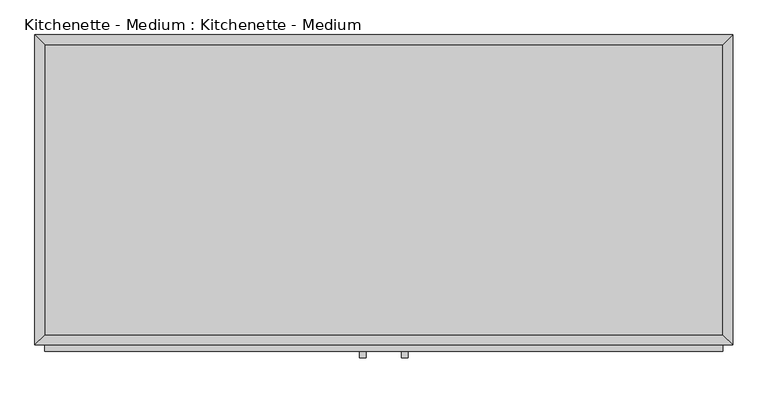
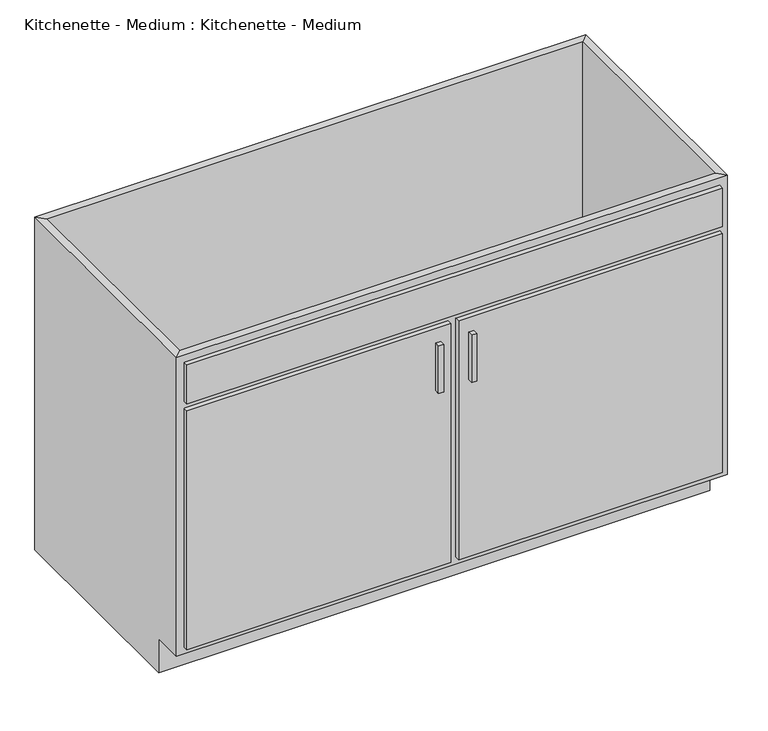
"""IFC4 building model written with IfcOpenShell, lengths in millimetres: proxy geometry, Kitchenette - Medium : Kitchenette - Medium."""

from ifc_helpers import new_model, si_unit, frame, origin, place, context, project, spatial, polyline, outline, extrude, faceted_brep, source, transform, mapped, element, save


def kitchenette_medium_kitchenette_medium_844211aa(model_context):
    return source(origin(), model_context, "Body", "SolidModel", [
        faceted_brep([(685.4877049, -590.55, 876.3), (685.4877049, -590.55, 88.9), (-648.0122951, -590.55, 88.9), (-648.0122951, -590.55, 876.3), (-667.0622951, -609.6, 876.3), (704.5377049, -609.6, 876.3), (-667.0622951, -609.6, 88.9), (704.5377049, -609.6, 88.9), (-648.0122951, -533.4, 88.9), (-648.0122951, -19.05, 88.9), (-648.0122951, -19.05, 876.3), (-667.0622951, 0.0, 876.3), (-667.0622951, 0.0, 0.0), (-667.0622951, -533.4, 0.0), (-667.0622951, -533.4, 88.9), (685.4877049, -19.05, 88.9), (685.4877049, -19.05, 876.3), (704.5377049, 0.0, 876.3), (704.5377049, 0.0, 0.0), (685.4877049, -533.4, 88.9), (704.5377049, -533.4, 88.9), (704.5377049, -533.4, 0.0)], [[[0, 1, 2, 3]], [[0, 3, 4, 5]], [[5, 4, 6, 7]], [[2, 1, 7, 6]], [[3, 2, 8, 9, 10]], [[4, 3, 10, 11]], [[6, 4, 11, 12, 13, 14]], [[2, 6, 14, 8]], [[10, 9, 15, 16]], [[11, 10, 16, 17]], [[12, 11, 17, 18]], [[1, 0, 16, 15, 19]], [[0, 5, 17, 16]], [[5, 7, 20, 21, 18, 17]], [[7, 1, 19, 20]], [[8, 19, 15, 9]], [[18, 21, 13, 12]], [[13, 21, 20, 19, 8, 14]]]),
        extrude(outline(polyline([(-16.1872951, -635.0), (-28.8872951, -635.0), (-28.8872951, -622.3), (-16.1872951, -622.3), (-16.1872951, -635.0)])), frame((0.0, 0.0, 573.769895), z_axis=(0.0, 0.0, 1.0), x_axis=(1.0, 0.0, 0.0)), (0.0, 0.0, 1.0), 124.730105),
        extrude(outline(polyline([(66.3627049, -635.0), (53.6627049, -635.0), (53.6627049, -622.3), (66.3627049, -622.3), (66.3627049, -635.0)])), frame((0.0, 0.0, 573.769895), z_axis=(0.0, 0.0, 1.0), x_axis=(1.0, 0.0, 0.0)), (0.0, 0.0, 1.0), 124.730105),
        extrude(outline(polyline([(685.4877049, -19.05), (685.4877049, -590.55), (-648.0122951, -590.55), (-648.0122951, -19.05), (685.4877049, -19.05)])), frame((0.0, 0.0, 88.9), z_axis=(0.0, 0.0, 1.0), x_axis=(1.0, 0.0, 0.0)), (0.0, 0.0, 1.0), 19.05),
        extrude(outline(polyline([(9.2127049, -622.3), (-648.0122951, -622.3), (-648.0122951, -609.6), (9.2127049, -609.6), (9.2127049, -622.3)])), frame((0.0, 0.0, 107.95), z_axis=(0.0, 0.0, 1.0), x_axis=(1.0, 0.0, 0.0)), (0.0, 0.0, 1.0), 628.65),
        extrude(outline(polyline([(685.4877049, -622.3), (28.2627049, -622.3), (28.2627049, -609.6), (685.4877049, -609.6), (685.4877049, -622.3)])), frame((0.0, 0.0, 107.95), z_axis=(0.0, 0.0, 1.0), x_axis=(1.0, 0.0, 0.0)), (0.0, 0.0, 1.0), 628.65),
        extrude(outline(polyline([(685.4877049, -622.3), (-648.0122951, -622.3), (-648.0122951, -609.6), (685.4877049, -609.6), (685.4877049, -622.3)])), frame((0.0, 0.0, 755.65), z_axis=(0.0, 0.0, 1.0), x_axis=(1.0, 0.0, 0.0)), (0.0, 0.0, 1.0), 101.6),
    ])


if __name__ == "__main__":
    model = new_model("IFC4")
    model_context = context("Model", 3, world=origin())
    ifc_project = project(units=[si_unit("LENGTHUNIT", "METRE", prefix="MILLI")], contexts=[model_context])
    site = spatial("IfcSite", under=ifc_project)
    building = spatial("IfcBuilding", under=site)
    placement = place(None, origin())
    kitchenette_medium_kitchenette_medium_shape = kitchenette_medium_kitchenette_medium_844211aa(model_context)
    element("IfcBuildingElementProxy", 1, Name="Kitchenette - Medium : Kitchenette - Medium", ObjectType="Kitchenette - Medium : Kitchenette - Medium", at=placement, inside=building, context=model_context, shape_type="MappedRepresentation", body=[
        mapped(kitchenette_medium_kitchenette_medium_shape, transform((0.0, 0.0, 0.0), x_axis=(1.0, 0.0, 0.0), y_axis=(0.0, 1.0, 0.0), z_axis=(0.0, 0.0, 1.0))),
    ])
    save(model, "model.ifc")

# Revit data of these elements
# Type "Kitchenette - Medium : Kitchenette - Medium"
#   Assembly Code = "E1090400"
#   Counter Length = 8' - 0"
#   Cabinet Width = 4' - 6"
#   Cabinet Height = 2' - 10 1/2"
#   Cabinet Depth = 2' - 0"
#   Toe Depth = 0' - 3"
#   Toe Height = 0' - 3 1/2"
#   Cabinet Material = Cabinets
#   Door/Drawer Material = Cabinets
#   Handle Material = Cabinets - Handles
#   Default Elevation = 0
# Element 1 (IfcBuildingElementProxy, "Kitchenette - Medium : Kitchenette - Medium")
#   Materials on its faces: "Cabinets", "Cabinets - Handles"
# Materials
#   "Cabinets": colour RGB 249 249 249, transparency 0
#   "Cabinets - Handles": class "Metal", colour RGB 57 57 57, transparency 0
